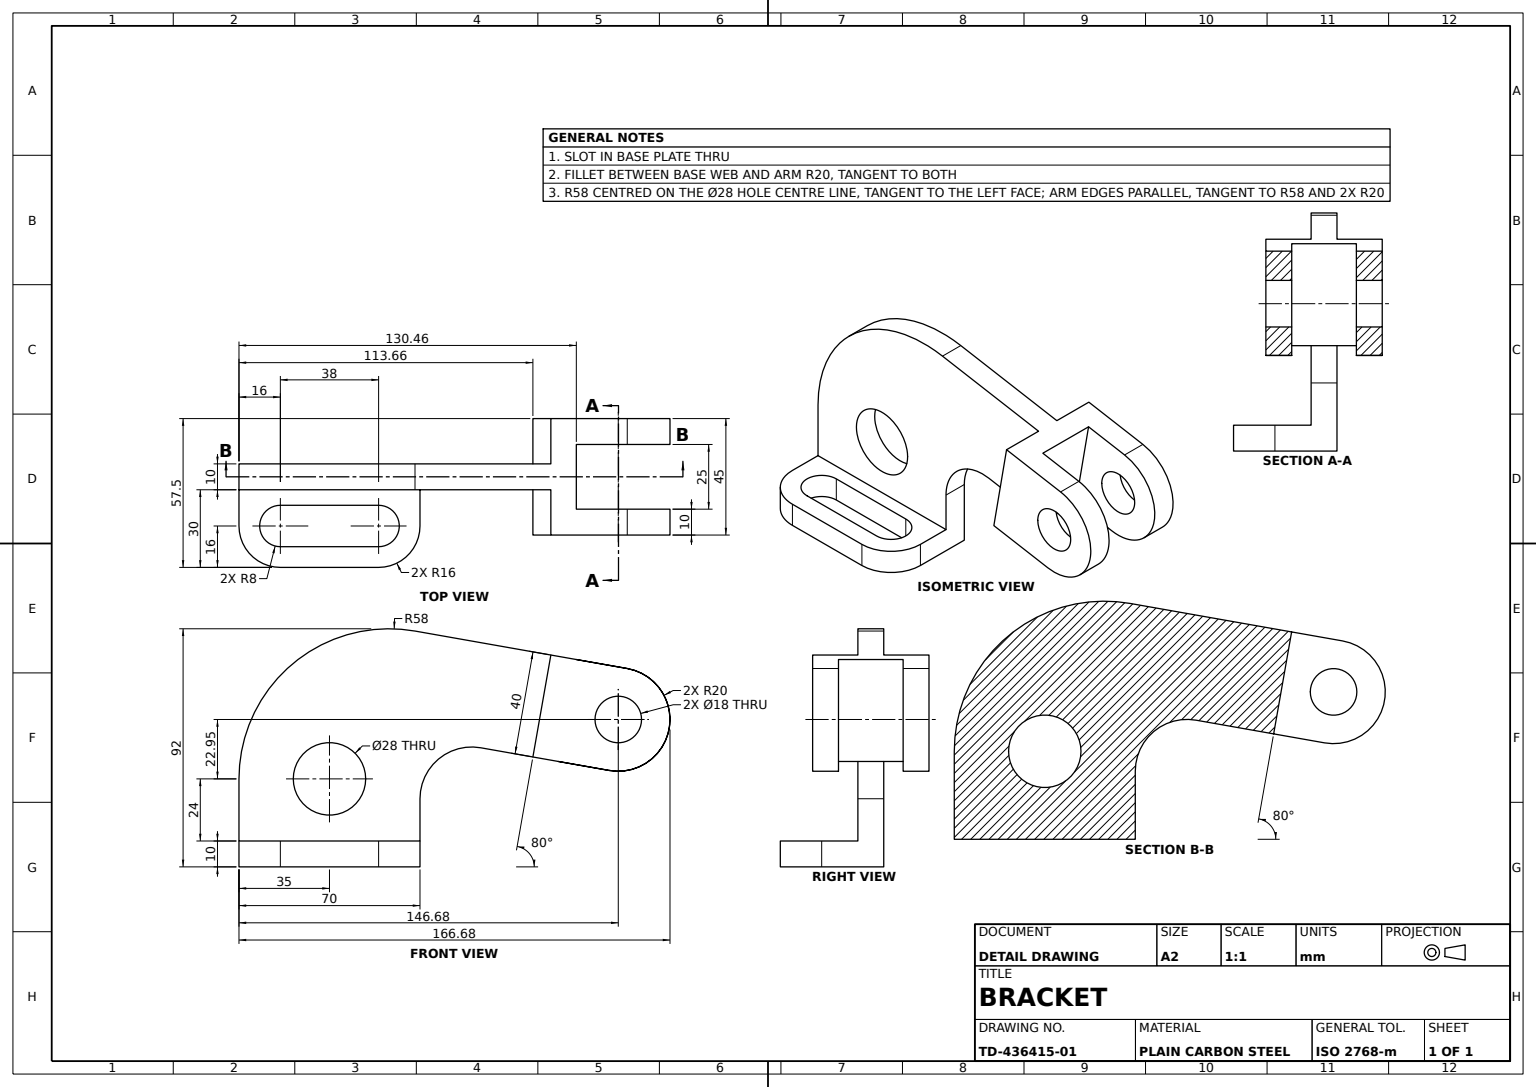
from build123d import *

# Parameters (mm, degrees)
SLOTTED_BASE_PLATE_DEPTH = 10
UPRIGHT_WEB_SKETCH_R     = 14
UPRIGHT_WEB_DEPTH        = 10
CLEVIS_ARM_DEPTH         = 40
CLEVIS_EAR_1_SKETCH_R    = 20
CLEVIS_EAR_1_DEPTH       = 10
CLEVIS_START             = -10
CLEVIS_EAR_2_SKETCH_R    = 20
CLEVIS_EAR_2_DEPTH       = 10
CLEVIS_PIN_HOLE_SKETCH_R = 9
CLEVIS_PIN_HOLE_18_DEPTH = 141.841641644


with BuildPart() as part:
    # Base Plate Sketch → Slotted Base Plate (new body)
    with BuildSketch(Plane(origin=(0, 0, 0), x_dir=(1, 0, 0), z_dir=(0, 1, 0))):
        with BuildLine():
            Line((0, 0), (-70, 0))
            Line((-70, 0), (-70, -14))
            ThreePointArc((-70, -14), (-65.313708499, -25.313708499), (-54, -30))
            Line((-54, -30), (-16, -30))
            ThreePointArc((-16, -30), (-4.686291501, -25.313708499), (0, -14))
            Line((0, -14), (0, 0))
        make_face()
        with BuildLine():
            Line((-54, -6), (-16, -6))
            ThreePointArc((-16, -6), (-8, -14), (-16, -22))
            Line((-16, -22), (-54, -22))
            ThreePointArc((-54, -22), (-62, -14), (-54, -6))
        make_face(mode=Mode.SUBTRACT)
    extrude(amount=SLOTTED_BASE_PLATE_DEPTH)

    # Upright Web Sketch → Upright Web (add)
    with BuildSketch(Plane(origin=(0, 0, 0), x_dir=(-1, 0, 0), z_dir=(0, 0, -1))):
        with BuildLine():
            Line((70, 0), (70, 34))
            ThreePointArc((70, 34), (49.281681362, 78.430577701), (1.928405695, 91.118849675))
            Line((1.928405695, 91.118849675), (-50.610518395, 81.85481982))
            Line((-50.610518395, 81.85481982), (-43.664591288, 42.4625097))
            Line((-43.664591288, 42.4625097), (-23.472963553, 46.022838454))
            ThreePointArc((-23.472963553, 46.022838454), (-7.144247806, 41.647572256), (0, 26.326683394))
            Line((0, 26.326683394), (0, 0))
            Line((0, 0), (70, 0))
        make_face()
        with Locations((35, 34)):
            Circle(UPRIGHT_WEB_SKETCH_R, mode=Mode.SUBTRACT)
    extrude(amount=UPRIGHT_WEB_DEPTH)

    # Clevis Arm Sketch → Clevis Arm (add)
    with BuildSketch(Plane(origin=(15.524092466, 88.041503368, 0), x_dir=(0.9848077530122072, -0.17364817766693494, 0), z_dir=(0.17364817766693494, 0.9848077530122072, 0))):
        Polygon((35.627690604, 27.5), (45.627690604, 27.5), (65.627690604, 27.5), (65.627690604, 17.5), (45.627690604, 17.5), (45.627690604, -7.5), (65.627690604, -7.5), (65.627690604, -17.5), (35.627690604, -17.5), align=None)
    extrude(amount=-CLEVIS_ARM_DEPTH)

    # Clevis Ear 1 Sketch → Clevis Ear 1 (add)
    with BuildSketch(Plane.XY.offset(17.5)):
        with Locations((76.681787432, 56.94921943)):
            Circle(CLEVIS_EAR_1_SKETCH_R)
    extrude(amount=-CLEVIS_EAR_1_DEPTH)

    # Clevis Ear 2 Sketch → Clevis Ear 2 (add)
    with BuildSketch(Plane(origin=(0, 0, -27.5), x_dir=(-1, 0, 0), z_dir=(0, 0, -1)).offset(CLEVIS_START)):
        with Locations((-76.681787432, 56.94921943)):
            Circle(CLEVIS_EAR_2_SKETCH_R)
    extrude(amount=CLEVIS_EAR_2_DEPTH)

    # Clevis Pin Hole Sketch → Clevis Pin Hole Ø18 (cut, through all)
    with BuildSketch(Plane.XY.offset(17.5)):
        with Locations((76.681787432, 56.94921943)):
            Circle(CLEVIS_PIN_HOLE_SKETCH_R)
    extrude(amount=-CLEVIS_PIN_HOLE_18_DEPTH, mode=Mode.SUBTRACT)


solid = part.part
